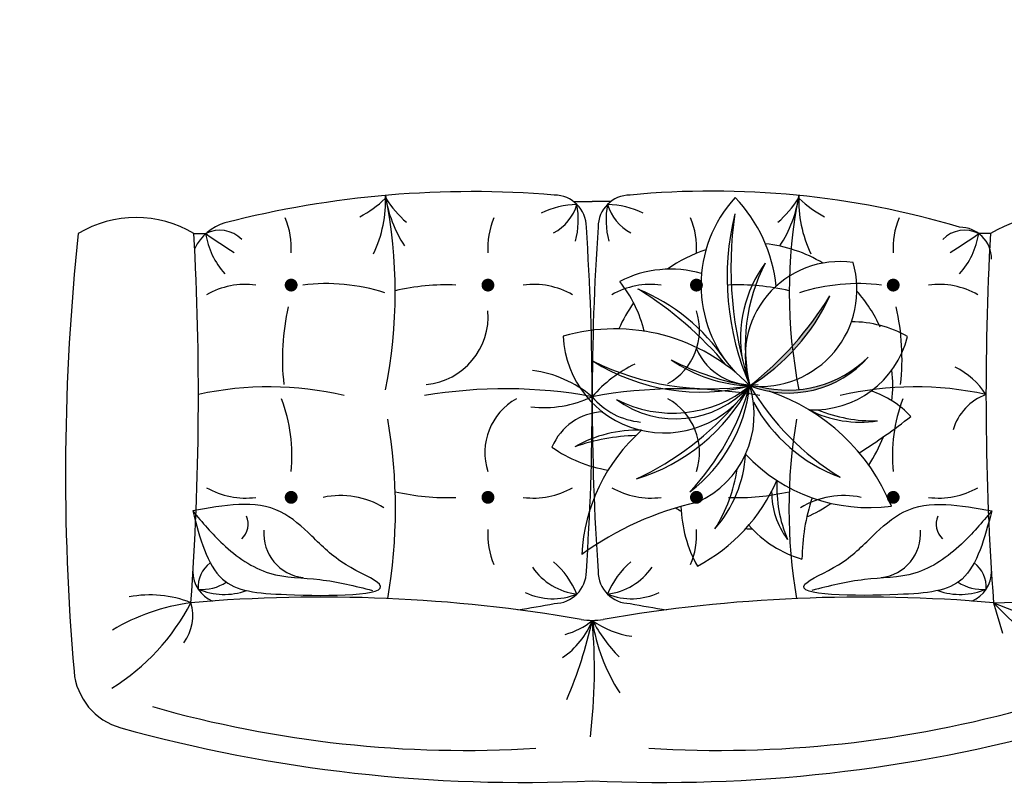
# Model space of a CAD drawing. Units: inches. Extents: x 844 to 2234, y 346 to 1084.
# Tile 67 of 93: x 1990 to 2014, y 669 to 688. Entities that reach past the tile are written whole.
import ezdxf

# ---------------------------------------------------------------- set-up
doc = ezdxf.new("R2010")
doc.units = ezdxf.units.IN
doc.header["$MEASUREMENT"] = 0
doc.layers.add('A-ANNO-DIMS', color=2, linetype='Continuous', lineweight=18)
doc.layers.add('furniture', color=8, linetype='Continuous', lineweight=18)
for name, color, linetype in [('RA-AP-01$0$FURN', 3, 'Continuous'), ('RA-AP-02$0$FLPT', 30, 'Continuous'), ('ROOM-NO', 3, 'Continuous')]:
    doc.layers.add(name, color=color, linetype=linetype)
doc.styles.get("Standard").update_dxf_attribs({"font": 'arial.ttf'})
doc.dimstyles.get("Standard").update_dxf_attribs({"dimtxt": 6, "dimasz": 3, "dimexe": 0.18, "dimexo": 0.0625, "dimgap": 0.09, "dimtad": 0, "dimtih": 1, "dimtoh": 1, "dimdec": 1, "dimzin": 0, "dimdsep": 46, "dimlunit": 3, "dimtxsty": 'Standard', "dimblk": 'ARCHTICK', "dimcen": 0.09, "dimadec": 0, "dimazin": 0, "dimtfac": 1, "dimtdec": 1, "dimtofl": 0, "dimtmove": 0, "dimatfit": 3, "dimfxl": 1, "dimtolj": 1, "dimtzin": 0, "dimarcsym": 0})

# ---------------------------------------------------------------- blocks, each defined once
blk = doc.blocks.new('A$C6E322C05')
at = {"layer": 'RA-AP-01$0$FURN'}
for p, q in [((6.391873508750865, -6.482044957760267), (6.516651486950081, -6.357266979564481)), ((6.391873508750865, -6.482044957760271), (6.43343929223883, -6.37746472106399)), ((6.391873508750866, -6.48204495776027), (6.390422568951521, -6.415535276369585)), ((6.391873508750865, -6.482044957760271), (6.439305270696451, -6.46824831830364)), ((5.817206456966433, -6.486712009544905), (5.817206456965108, -6.505053364959449)), ((5.767206456949363, -7.077520703653457), (5.767206456948565, -7.10671200954539)), ((5.767206456949363, -7.135903315437323), (5.767206456948565, -7.10671200954539)), ((5.817206456966433, -7.726712009545875), (5.817206456965108, -7.70837065413133))]:
    blk.add_line(p, q, dxfattribs=at)
at = {"layer": 'RA-AP-01$0$FURN', "const_width": 0.01}
for points in [[(5.902459393885763, -6.638129816788149, 1), (5.892459393885761, -6.638129816788122, 1)], [(6.222844373610339, -6.638129816788595, -1), (6.23284437361034, -6.638129816788595, -1)], [(5.902459393885763, -6.944444251846759, -1), (5.892459393885761, -6.944444251846785, -1)], [(6.222844373610339, -6.944444251846313, 1), (6.23284437361034, -6.944444251846313, 1)], [(5.902459393885763, -7.268979767244021, 1), (5.892459393885761, -7.268979767243994, 1)], [(6.222844373610339, -7.268979767244466, -1), (6.23284437361034, -7.268979767244466, -1)], [(5.902459393885763, -7.575294202302631, -1), (5.892459393885761, -7.575294202302657, -1)], [(6.222844373610339, -7.575294202302185, 1), (6.23284437361034, -7.575294202302185, 1)]]:
    blk.add_lwpolyline(points, format="xyb", close=True, dxfattribs=at)
at = {"layer": 'RA-AP-01$0$FURN'}
for centre, radius, start, end in [((6.192206456970573, -9.839674509409203), 3.552808610866049, 85.0473312316412, 96.0588723756579), ((5.962206456956505, -6.396712009545393), 0.1706604816468166, 148.1725534208377, 211.8274465791593), ((6.490296991311982, -6.399757455669855), 0.1, 15.49949460085664, 85.04733123164101), ((4.33669785707999, -6.99698289606033), 2.33487526667919, 357.3063521928599, 15.49949460085664), ((4.846593614069285, -6.909687157115225), 1.775196618325768, 356.4780136403396, 15.93354743557553), ((6.068281987477935, -2.019830784287151), 4.473931917517753, 266.7828902523826, 274.1477233631118), ((8.747044799885572, -6.68548500417652), 2.363941552380466, 175.0630368065897, 189.8434409139549), ((5.857266904022845, -6.534972599266733), 0.05, 90.00000000094654, 180), ((6.134026645419561, -6.595486433826224), 0.1214600988114338, 123.1053299945123, 153.7006015369794), ((6.565877894706778, -6.603111116245941), 0.5100538472773755, 167.6182489359307, 193.3122231353938), ((6.14746341585187, -6.463466129962243), 0.0853281020358404, 200.7831020638199, 253.0462459140071), ((6.367926665937501, -6.54114871013533), 0.0478550828899777, 86.575295631534, 142.6833829238214), ((6.343036863464309, -6.534972599266733), 0.05, 22.58267242460392, 89.99999999905346), ((6.302747869360707, -6.499593011892033), 0.0683206773889159, 326.6729861493449, 5.218395042636973), ((6.274768375315671, -6.53387763124781), 0.1042084262671507, 340.4828318717155, 22.86929393278168), ((5.860011614985668, -6.526983908613928), 0.0479292786975047, 152.8070868543555, 225.4025460716553), ((5.798239671935704, -6.625433523557484), 0.1218651776285568, 48.0375529564433, 81.0462320954125), ((4.904259194880517, -7.136565421857206), 1.11020813118073, 31.93286085977143, 34.66647731879807), ((6.017778833798976, -6.566879816788349), 0.1214118203512435, 150.1419074485596, 187.691663289156), ((6.107524933697323, -6.566879816788473), 0.1214118203512435, 352.3083367106845, 29.85809255128089), ((7.09459581372041, -6.919286936999045), 1.343470592134322, 163.3777289595395, 185.4806594039327), ((6.269780256940199, -6.54020363968894), 0.0310151388417235, 245.7760318513891, 317.3789451550392), ((6.284290296802319, -6.664490968717984), 0.0689028341546707, 6.419517109091462, 94.46157264568865), ((5.839565409091811, -6.517091257029312), 0.1212957045587361, 247.3375839744822, 273.7314750942433), ((6.011601695098697, -6.976164478788355), 0.3517162425384579, 83.41248966761121, 103.1674570565571), ((6.162348040003244, -6.395238182300004), 0.2442261434243043, 248.9017070735605, 275.9923925191661), ((6.197523316847625, -6.692545952238853), 0.3023568492824586, 173.0944825511667, 197.588060785551), ((6.354517986346992, -6.715077923337803), 0.1295083186917369, 167.9901339202812, 211.3796151021958), ((5.650260521516567, -6.673548227893377), 0.1579426672576338, 315.4052081938554, 333.0844958846701), ((5.765922189292775, -6.593612516654137), 0.1915923630277471, 267.5852697713958, 295.5830728418392), ((5.908792452070163, -6.03459657477793), 0.765467899454341, 258.6273206109321, 281.4174148186357), ((5.73314461686815, -6.969744817001631), 0.1863549309199891, 56.29262493376822, 82.3818003344588), ((5.679375702373212, -6.920075501166131), 0.1579426672576338, 40.38651175517922, 58.06579944599388), ((6.245858341704271, -5.977214432993086), 0.8232838708255751, 260.2449188973366, 279.7550811026635), ((6.245792934290092, -6.879444251846194), 0.3486563571350461, 166.839178360846, 182.4657575311016), ((5.879510833205829, -6.879444251846704), 0.3486563571350461, 357.5342424690579, 13.1608216393135), ((5.959527339947079, -6.859074294904489), 0.0930420630931112, 293.6025128512426, 6.610683813350465), ((6.80739198570858, -6.9716011229856), 0.7485435294774117, 170.3094183042209, 190.3986311369044), ((5.967289987028921, -7.035039638983766), 0.0953802309589454, 28.80342840007747, 108.2253060204472), ((6.158013780467433, -7.035039638983501), 0.0953802309589454, 71.7746939797123, 151.196571600082), ((5.839565409091811, -7.065482811605596), 0.1212957045587361, 86.2685249057567, 112.6624160255178), ((6.285738358404627, -7.065482811604976), 0.1212957045587361, 67.33758397464167, 93.73147509440282), ((6.017778833798976, -7.015694251846559), 0.1214118203512435, 172.308336710844, 209.8580925514404), ((6.107524933697323, -7.015694251846435), 0.1214118203512435, 330.1419074487191, 7.691663289315497), ((6.286338558013386, -7.045586518350251), 0.0993499474027353, 337.9047121936679, 25.63436525513283), ((5.08702348459791, -6.791287034316994), 1.330927509443381, 348.8964178164725, 351.3771209523497), ((6.280014948979332, -7.094901076442985), 0.0990996950214925, 6.922564260119504, 55.10883789097723), ((5.904234274973987, -7.085727051545815), 0.1323517050571434, 153.8887786398558, 178.8006589660143), ((5.999456242224805, -7.021102361717039), 0.1116589361851176, 309.9425663137084, 354.6905921774272), ((5.807266904022846, -7.047601469367252), 0.05, 180, 269.9999999990534), ((5.751472800077547, -7.013313769593298), 0.07258027258109, 286.3558526771587, 332.6774804096085), ((6.211136556040091, -6.947122539501678), 0.212288550941915, 205.9704430982785, 228.7419974602242), ((6.4323439288987, -6.955317466880212), 0.1385734111998875, 221.2288777133949, 247.0867614897648), ((6.343036863466045, -7.047601469376512), 0.05, 269.9999999989608, 359.9999999989431), ((6.304557655687245, -7.024767404076127), 0.1410608784479501, 324.4849629611242, 351.797284145529), ((6.374625390672053, -6.818147225624045), 0.2920141296149301, 278.8152064253152, 302.6921045175205), ((6.285596300104752, -6.865193601455727), 0.2760944594998999, 298.9825510110601, 313.6694461006315), ((5.795585623761384, -6.952739633017071), 0.1323517050571434, 259.6959164764198, 284.6077968025783), ((6.319376003798462, -7.10671200954539), 0.1, 350.1565590860452, 9.843440913955273), ((6.075151883811576, -3.163731520221818), 3.942980489323571, 266.1043400737264, 273.8956599242929), ((6.075151883808545, -11.04969249895812), 3.942980489412734, 86.10434007575122, 93.89565992614118), ((6.213892115887508, -7.225151532818968), 0.1854874288882049, 140.3167953258794, 172.0522897837384), ((6.80739198570858, -7.241822896105179), 0.7485435294774117, 169.6010516837189, 189.690581695779), ((5.911254573522987, -7.182496879996349), 0.1769409696162427, 353.679636560008, 25.3608296845614), ((6.496371549498975, -7.961935855380467), 0.8586827939016008, 83.03755924582121, 95.14445252709366), ((6.375720249476352, -7.220682794696101), 0.1220457486080966, 33.71356548940426, 69.04099283815023), ((6.338324584842819, -7.175279287582296), 0.1061640434993627, 14.36483859718907, 40.23030537468725), ((6.269502792941208, -7.789055933740261), 0.6986094833441214, 67.00911261779231, 77.61200156369726), ((4.336697857080025, -7.216441123030454), 2.334875266679154, 344.5005053991432, 2.69364780714023), ((5.807266904022846, -7.165822549723527), 0.05, 90.00000000094654, 180), ((6.343036863466045, -7.165822549714267), 0.05, 1.0568602e-09, 90.00000000103913), ((8.747044799885572, -7.527939014914259), 2.363941552380466, 170.156559086045, 184.9369631934102), ((5.795585623761384, -7.260684386073708), 0.1323517050571434, 75.39220319742172, 100.3040835235802), ((5.904234274973987, -7.127696967544965), 0.1323517050571434, 181.1993410339857, 206.1112213601442), ((5.751472800077547, -7.200110249497481), 0.07258027258109, 27.32251959039153, 73.64414732284132), ((6.017778833798976, -7.19772976724422), 0.1214118203512435, 150.1419074485596, 187.691663289156), ((6.107524933697323, -7.197729767244345), 0.1214118203512435, 352.3083367106845, 29.85809255128088), ((6.4323439288987, -7.25810655221026), 0.1385734111998875, 112.9132385102352, 138.7711222866051), ((6.280014948979332, -7.118522942647487), 0.0990996950214925, 304.8911621090228, 353.0774357398805), ((6.286338558013386, -7.167837500740221), 0.0993499474027353, 334.3656347448672, 22.09528780633203), ((7.290981934450236, -7.293982589837588), 1.539060359583382, 175.2233567466078, 194.4661216781742), ((5.08702348459791, -7.422136984773786), 1.330927509443381, 8.62287904765033, 11.10358218352746), ((4.846593614069285, -7.303736861975558), 1.775196618325768, 344.0664525644245, 3.521986359660393), ((6.158013780467433, -7.178384380107278), 0.0953802309589454, 208.803428399918, 288.2253060202877), ((5.839565409091811, -7.147941207485184), 0.1212957045587361, 247.3375839744822, 273.7314750942433), ((6.285738358404627, -7.147941207485803), 0.1212957045587361, 266.2685249055972, 292.6624160253583), ((5.946346035540796, -7.374645549675604), 0.1060388135390937, 5.185910074000148, 94.80734315124221), ((6.245792934290092, -7.333979767244585), 0.3486563571350461, 177.5342424688983, 193.160821639154), ((5.879510833205829, -7.333979767244075), 0.3486563571350461, 346.8391783606865, 2.465757530942165), ((5.73314461686815, -7.243679202089149), 0.1863549309199891, 277.6181996655412, 303.7073750662318), ((5.679375702373212, -7.293348517924648), 0.1579426672576338, 301.9342005540061, 319.6134882448208), ((5.908792452070163, -8.17882744431285), 0.765467899454341, 78.58258518136427, 101.3726793890678), ((6.245858341704271, -8.236209586097694), 0.8232838708255751, 80.24491889733653, 99.75508110266345), ((5.765922189292775, -7.619811502436642), 0.1915923630277471, 64.41692715816083, 92.41473022860427), ((5.650260521516567, -7.539875791197403), 0.1579426672576338, 26.91550411532996, 44.59479180614462), ((6.197523316847625, -7.520878066851927), 0.3023568492824586, 162.411939214449, 186.9055174488332), ((6.354517986346992, -7.498346095752976), 0.1295083186917369, 148.6203848978042, 192.0098660797188), ((6.565877894706778, -7.610312902844838), 0.5100538472773755, 166.6877768646062, 192.3817510640693), ((6.284290296802319, -7.548933050372795), 0.0689028341546707, 265.5384273543114, 353.5804828909086), ((5.839565409091811, -7.696332762061468), 0.1212957045587361, 86.26852490575668, 112.6624160255178), ((6.011601695098697, -7.237259540302424), 0.3517162425384579, 256.8325429434429, 276.5875103323888), ((6.162348040003244, -7.818185836790775), 0.2442261434243043, 84.00760748083387, 111.0982929264395), ((6.017778833798976, -7.646544202302431), 0.1214118203512435, 172.308336710844, 209.8580925514404), ((6.107524933697323, -7.646544202302306), 0.1214118203512435, 330.1419074487191, 7.691663289315504), ((6.269780256940199, -7.67322037940184), 0.0310151388417235, 42.62105484496073, 114.2239681486109), ((6.274768375315671, -7.679546387842969), 0.1042084262671507, 337.1307060672183, 19.51716812828453), ((5.860011614985668, -7.686440110476851), 0.0479292786975047, 134.5974539283447, 207.1929131456445), ((4.904259194880517, -7.076858597233573), 1.11020813118073, 325.333522681202, 328.0671391402286), ((6.302747869360707, -7.713831007198747), 0.0683206773889159, 354.781604957363, 33.32701385065516), ((5.87316911435942, -7.657653239374848), 0.0753785023123622, 196.0166452769965, 244.1254380939442), ((5.798239671935704, -7.587990495533295), 0.1218651776285568, 278.9537679045876, 311.9624470435567), ((6.367926665937501, -7.672275308955449), 0.0478550828899777, 217.3166170761785, 273.424704368466), ((6.343036863464309, -7.678451419824046), 0.05, 270.0000000009465, 337.4173275753961), ((6.068281987477935, -12.19359323480363), 4.473931917517753, 85.85227663688822, 93.21710974761734), ((5.966706456956126, -7.816712009545387), 0.1744999999876311, 148.9517780040469, 211.0482219959533), ((6.549562589740832, -7.794613830093475), 0.1698955038956699, 158.1487616198804, 191.122156864055), ((6.412319729336772, -7.798818772412041), 0.0704710051510922, 53.58735038429053, 106.8661365794674), ((6.713110001951175, -7.687961227420911), 0.3241573581843151, 187.6973649013944, 210.7014325157311), ((6.237117433414106, -8.032110101276656), 0.3382138395168437, 31.74362916573515, 62.76966729059727), ((6.49029699131198, -7.813666563420925), 0.1, 274.9526687683584, 344.500505399143), ((6.192206456970577, -4.373749509681577), 3.552808610866049, 263.941127624342, 274.9526687683587)]:
    blk.add_arc(centre, radius, start, end, dxfattribs=at)
for points, knots in [([(6.249068123947751, -6.484897777661085), (6.239897409094627, -6.533353418276971), (6.226611264288107, -6.603553906267942), (6.290696373977354, -6.673990528916563), (6.332121563214334, -6.713363084361603), (6.381789098403072, -6.831232979612737), (6.381738454094183, -6.629656072516828), (6.370771929626907, -6.516634365426866), (6.291185937762818, -6.495880800642047), (6.249068123947751, -6.484897777661087)], [0, 0, 0, 0, 0.1367586589314792, 0.1981301758052368, 0.2677729570689282, 0.3281194902553322, 0.4737578340741565, 0.5765194025309516, 0.6920332287422236, 0.6920332287422236, 0.6920332287422236, 0.6920332287422236]), ([(6.249068123947751, -6.484897777661087), (6.266851662635476, -6.499857019491296), (6.306238891621481, -6.532988956490432), (6.353826300430336, -6.600137645661404), (6.352465874908733, -6.685122080531377), (6.365878290565239, -6.737689715716581), (6.372748706337224, -6.764617117843226)], [0, 0, 0, 0, 0.070018540671015, 0.1550780383534498, 0.2344491945777043, 0.3178048737568289, 0.3178048737568289, 0.3178048737568289, 0.3178048737568289]), ([(6.249068123947751, -7.728526241429694), (6.239897409094627, -7.680070600813808), (6.226611264288107, -7.609870112822835), (6.290696373977354, -7.539433490174218), (6.332121563214334, -7.500060934729178), (6.381789098403072, -7.382191039478041), (6.381738454094183, -7.583767946573952), (6.370771929626907, -7.696789653663914), (6.291185937762818, -7.717543218448732), (6.249068123947751, -7.728526241429692)], [0, 0, 0, 0, 0.1367586589314792, 0.1981301758052368, 0.2677729570689282, 0.3281194902553322, 0.4737578340741565, 0.5765194025309516, 0.6920332287422236, 0.6920332287422236, 0.6920332287422236, 0.6920332287422236]), ([(6.249068123947751, -7.728526241429692), (6.266851662635476, -7.713566999599485), (6.306238891621481, -7.680435062600349), (6.353826300430336, -7.613286373429378), (6.352465874908733, -7.528301938559401), (6.365878290565239, -7.475734303374198), (6.372748706337224, -7.448806901247554)], [0, 0, 0, 0, 0.070018540671015, 0.1550780383534498, 0.2344491945777043, 0.3178048737568289, 0.3178048737568289, 0.3178048737568289, 0.3178048737568289])]:
    blk.add_open_spline(points, degree=3, knots=knots, dxfattribs=at)
blk = doc.blocks.new('A$C78016F37')
at = {"layer": 'RA-AP-02$0$FLPT'}
for points in [[(8.585816203069419, -6.02390819987247, -0.263770389754008), (8.460672408962632, -5.900531828839305, -0.0241291823863587), (8.454072418949808, -5.887595694471202, 2.53684562776e-05), (8.45404743172537, -5.887630207283394, 0.3135010205465867)], [(8.6375288720004, -5.923949758415821, -0.0887687358956854), (8.454121692088984, -5.887527659105068, 7.7903089823e-06), (8.45411401635844, -5.887538255716633, 0.1521261679004899)]]:
    blk.add_hatch(color=256, dxfattribs=at).paths.add_polyline_path(points)
at = {"layer": 'RA-AP-01$0$FURN'}
for centre, radius, start, end in [((8.676215054199671, -5.667660989702041), 0.3125591380039201, 178.1117989109854, 224.6938723266582), ((8.77416640415315, -5.62926868308301), 0.4113013577889528, 183.916601998098, 218.889069239545), ((8.454024671827373, -5.887489670112504), 0.2224048992971994, 84.85146405771819, 96.8968759960221), ((7.926806489084671, -5.648344237112944), 0.5693232143741963, 340.3683676450975, 358.6332230039188), ((8.195746570571197, -5.703566525505195), 0.3030929277970076, 334.410018118324, 8.056842366720524), ((8.454024671827373, -5.887489670112504), 0.2224048992971994, 48.29632106119188, 65.66234443375417), ((8.028579057188336, -5.942548842808446), 0.3176725093823991, 32.12276904396682, 49.65676958807643), ((8.138392155386812, -5.868774225710474), 0.1937166188785145, 28.24647600965292, 60.3482035660113), ((8.485489110864293, -5.735116799889917), 0.1555876039528135, 173.9896977683083, 258.3326220930856), ((8.521327457039675, -5.708924385009453), 0.1908277389198635, 182.9741757068071, 249.3481441545862), ((8.654249619708994, -5.778555799161595), 0.2279399438329033, 175.7401143551485, 208.5487298435666), ((8.841321835932057, -5.738299260526738), 0.4150383977849519, 183.2217031044116, 201.067141094303), ((8.442163868805496, -5.589503946884691), 0.2981456377964393, 227.2393731923049, 272.0875214538299), ((8.499731284894388, -5.433816546692462), 0.4559697329776795, 235.2365058162176, 260.2774785796924), ((8.454024671827373, -5.887489670112504), 0.2224048992971994, 359.5998786150253, 24.14255533511359), ((8.645911592327788, -6.090477518425219), 0.27932894017942, 93.04938662579335, 133.3896949469156), ((8.610008543493892, -6.006599373458567), 0.1961871509349957, 83.84242350983102, 130.6121505715144), ((8.564547574985227, -5.985184712735347), 0.1475114689626245, 22.41040215178937, 138.5254141817128), ((8.454024671827373, -5.887489670112504), 0.2224048992971994, 179.1222698891959, 181.6416201752811), ((8.343226438185093, -5.786283478281637), 0.1500631261941314, 234.481997856841, 317.590554229248), ((8.35533458686642, -5.671200371653297), 0.2372928460263133, 247.4602721701189, 294.3106346998744), ((8.353310301606033, -5.50080131865886), 0.3995888706145134, 257.1400840392136, 284.5985568218482), ((8.820839898988444, -6.089372712149781), 0.4186128907603021, 151.1845644972185, 178.7925181665867), ((8.647592804319403, -5.39327801538501), 0.5307671632505924, 248.6111860886518, 268.9135435570199), ((8.591324349397098, -5.825721750746069), 0.1505539017216363, 204.2218678925879, 316.713948440902), ((8.60427433017431, -5.61130057980146), 0.3144127437625546, 241.4533621372112, 276.0713675084609), ((8.617925276426345, -5.861018191689067), 0.1660245384207697, 189.1745772070899, 258.8487542743241), ((8.650970463531563, -6.036034461900849), 0.252604074752176, 148.7548044074418, 190.1503402437527), ((8.632043935228618, -5.851861780578565), 0.1781487401371014, 195.8547118906642, 254.9602254039967), ((8.27103219642381, -5.762377687346963), 0.1942058542978326, 259.1738264472347, 296.9361074578899), ((8.242487148295718, -5.713440208635033), 0.2398180026482373, 268.1044384936476, 291.9165885710061), ((8.454024671827373, -5.887489670112504), 0.2224048992971994, 324.5751954876287, 341.8360454133948), ((8.643418645519843, -5.97565241718072), 0.1753165964770544, 183.2000241261284, 219.1319783506275), ((8.454024671827373, -5.887489670112504), 0.2224048992971994, 208.6999597596628, 211.2898901048327), ((8.447576280134497, -6.186493140077375), 0.2128537218708566, 117.7922244992203, 143.1680179163233), ((8.391080266506174, -6.106601067273632), 0.1233275614230441, 120.0065551025349, 157.0200898875673), ((8.702436309821351, -5.965526387054176), 0.2293777808440535, 187.970132899875, 211.770006950379), ((8.454024671827373, -5.887489670112504), 0.2224048992971994, 233.8814212202215, 245.0364073377333), ((8.454024671827373, -5.887489670112504), 0.2224048992971994, 294.3332330132876, 306.7022905924929), ((8.454024671827373, -5.887489670112504), 0.2224048992971994, 266.6746775461067, 279.4836973606225)]:
    blk.add_arc(centre, radius, start, end, dxfattribs=at)
at = {"layer": 'RA-AP-02$0$FLPT'}
blk.add_lwpolyline([(8.373681407360612, -5.597603282219753, 0.7334826821515817), (8.454024671827373, -5.887489670112506, 0.2766279680881699), (8.373681407360612, -5.597603282219752, 1.3559471233864)], format="xyb", dxfattribs=at)
for centre, radius, start, end in [((8.307234168263015, -5.560224752275053), 0.1974581866646199, 313.6950443365965, 339.1517930721081), ((8.39717548070647, -5.778250590985688), 0.1754354389711152, 14.56900959352841, 57.37320031926483), ((8.423880035729836, -5.687934118592295), 0.2086915776254087, 175.0742803806306, 201.2122531761669), ((8.228139151249446, -5.75774524127399), 0.0885717136803359, 32.28640253436571, 97.90409188948885), ((8.433135668112254, -6.051756800567661), 0.1760533926534347, 161.4400574260173, 193.8427700955681), ((8.41746442128814, -6.364284642428606), 0.3118134108627832, 101.9980156162763, 119.8647524560376), ((8.395985399479063, -6.084837299933293), 0.1497734353479364, 343.3485825573843, 11.74756506179821), ((8.942045887600607, -5.120169675385827), 1.085029101271162, 243.0359441902965, 248.2214525024466)]:
    blk.add_arc(centre, radius, start, end, dxfattribs=at)
at = {"layer": 'ROOM-NO'}
for centre, radius, start, end in [((8.65235909715731, -5.915275987506324), 0.2002713751519826, 77.61332513631854, 163.1649854687259), ((8.897731643814414, -6.279909663508004), 0.5923422390868573, 112.2662452820337, 138.5100534847894), ((8.794175340646271, -6.133856003178959), 0.4198977696908007, 106.7322927724504, 144.0984247900076), ((8.46944987509335, -5.65497750757116), 0.2349499976215632, 306.2836330402241, 344.0182681768919), ((8.22288024947718, -6.040653787747125), 0.2772850355038946, 71.89678357893693, 117.3860017964977), ((7.898132843717886, -6.242790504972724), 0.48979813475044, 43.05187184217114, 66.25811984072557), ((8.347851773195234, -6.064576052783105), 0.2064758371609359, 122.2147792747386, 149.2270256684313), ((8.154124515379644, -5.981454547332234), 0.314276155615234, 322.6594768637323, 11.71644421186061), ((8.609526443069848, -6.010438452646774), 0.261483616160276, 163.3494523104177, 218.1824089018609), ((8.3154997513214, -5.724318991124441), 0.2758350084868725, 238.2734303421065, 276.8355613505966), ((8.468611314717652, -6.062483436674201), 0.1756006505860901, 0.6277371554985871, 30.43990742705027), ((8.602078464955955, -5.915823919619132), 0.1507406891149966, 207.5045866236536, 286.2267783265413)]:
    blk.add_arc(centre, radius, start, end, dxfattribs=at)
blk = doc.blocks.new('A$C5D2F253E')
at = {"layer": 'RA-AP-01$0$FURN', "xscale": -1}
blk.add_blockref('A$C6E322C05', (4.620200485489021, 7.961130550668883), dxfattribs=at)
at = {"layer": 'RA-AP-02$0$FLPT', "xscale": -1, "rotation": 210.3787734063952}
blk.add_blockref('A$C78016F37', (-5.749960471669055, -8.254610923396115), dxfattribs=at)
blk = doc.blocks.new('_ArchTick')
at = {"color": 0, "linetype": 'ByBlock', "const_width": 0.15}
blk.add_lwpolyline([(-0.5, -0.5), (0.5, 0.5)], dxfattribs=at)
blk = doc.blocks.new('*D121')
at = {"layer": 'A-ANNO-DIMS', "color": 0, "lineweight": -2, "transparency": 16777216}
for p, q in [((2030.271987351997, 734.262611118704), (2040.245275089302, 734.262611118704)), ((2040.065275089302, 734.262611118704), (2040.065275089302, 704.6043509484256)), ((2040.065275089302, 668.557359536674), (2040.065275089302, 698.2156197069523)), ((2030.271987351997, 668.557359536674), (2040.245275089302, 668.557359536674))]:
    blk.add_line(p, q, dxfattribs=at)
at = {"layer": 'Defpoints', "color": 0, "transparency": 16777216}
for p in [(2030.209487351997, 734.262611118704), (2040.065275089302, 734.262611118704), (2030.209487351997, 668.557359536674)]:
    blk.add_point(p, dxfattribs=at)
at = {"layer": 'A-ANNO-DIMS', "color": 0, "lineweight": -2, "transparency": 16777216, "xscale": 3, "yscale": 3, "zscale": 3}
for p, rotation in [((2040.065275089302, 734.262611118704), 90), ((2040.065275089302, 668.557359536674), 270)]:
    blk.add_blockref('_ArchTick', p, dxfattribs=dict(at, rotation=rotation))
at = {"layer": 'A-ANNO-DIMS', "color": 0, "transparency": 16777216, "insert": (2040.065275089302, 701.4099853276883), "char_height": 6, "attachment_point": 5}
blk.add_mtext('\\A1;LOUNGE SET 5\'-5 1/2" TYP.', dxfattribs=at)

msp = doc.modelspace()

# ---------------------------------------------------------------- block references
at = {"layer": 'furniture', "xscale": -15.94108302203742, "yscale": 15.94108302203742, "zscale": 15.94108302203742, "rotation": 270}
msp.add_blockref('A$C5D2F253E', (1990.567271852805, 701.4028671565849), dxfattribs=at)

# ---------------------------------------------------------------- dimensions: what is measured, and where the dimension line sits
at = {"layer": 'A-ANNO-DIMS'}
dim = msp.add_linear_dim(base=(2040.065275089302, 734.262611118704), p1=(2030.209487351996, 668.5573595366737), p2=(2030.209487351996, 734.2626111187037), angle=90, text='LOUNGE SET <> TYP.', dimstyle='Standard', override={"dimdec": 1, "dimlfac": 1, "dimrnd": 0, "dimzin": 1, "dimdsep": 46, "dimlunit": 4, "dimfrac": 2}, dxfattribs=at)
dim.commit()
dim.dimension.update_dxf_attribs({"geometry": '*D121', "text_midpoint": (2040.065275089302, 701.4099853276883)})

doc.saveas('drawing.dxf')
